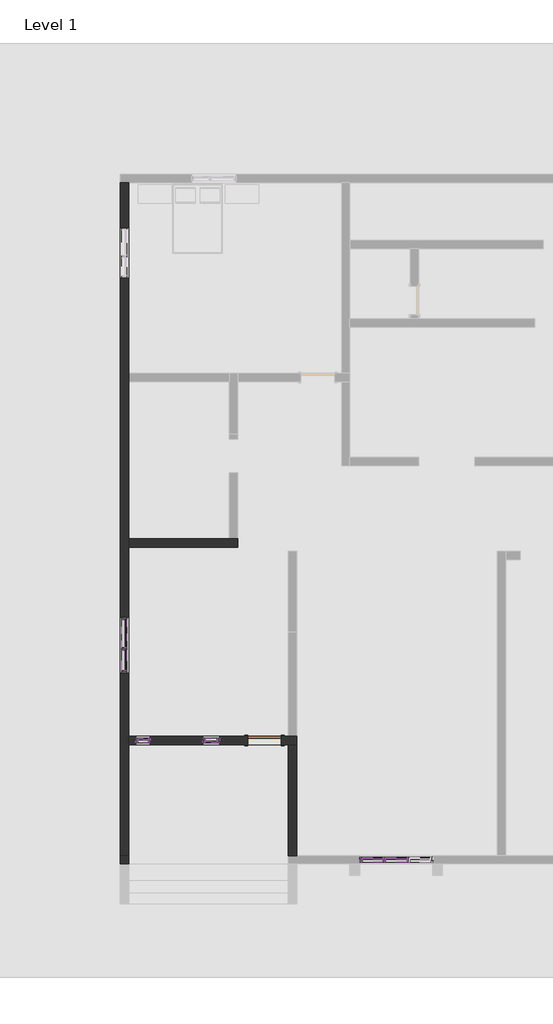
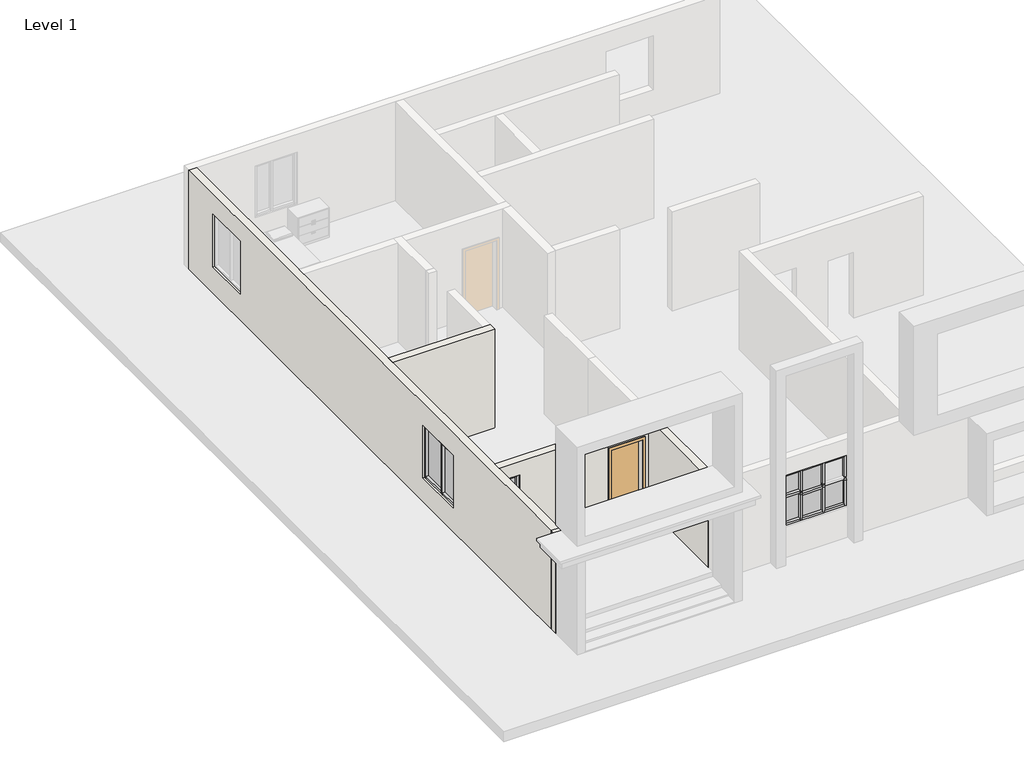
# One storey, part 1 of 3: 50 members, 13 plates, 5 walls, 1 door.
"""IFC4 building model written with IfcOpenShell, lengths in millimetres."""

from ifc_helpers import new_model, si_unit, origin, origin_with_axes, place, context, project, spatial, polyline, outline, extrude, faceted_brep, transform, mapped, element, save
from components import door_0ca8825f, member_d3323a85, member_6be37683, member_b3e70a48, member_ff9f2d30, member_0c1408be, member_6f814c25, member_392009c2, member_a2013922, member_4a5c7385, member_495a21e7, member_6f432376, member_6103f85b, member_d3f030c1, member_3af75de8, member_a400357f, member_b527cf9c, member_e59bf7ef, member_86293703, member_46f5bc36, member_037f74fd, member_7862cfa9, system_panel_glazed_ef88186a, system_panel_glazed_df0efb0a, system_panel_glazed_3a0990d6, system_panel_glazed_e5302343, system_panel_glazed_871766ed, system_panel_glazed_cbb2ce41, system_panel_glazed_89c3752f, system_panel_glazed_000d40f8, system_panel_glazed_6bcf57a8, system_panel_glazed_fab24249, system_panel_glazed_9a45502e

model = new_model("IFC4")

# Units and contexts
model_context = context("Model", 3, world=origin())
ifc_project = project(units=[si_unit("LENGTHUNIT", "METRE", prefix="MILLI")], contexts=[model_context])

# Site, building, storey
site = spatial("IfcSite", under=ifc_project)
building = spatial("IfcBuilding", under=site)
storey = spatial("IfcBuildingStorey", under=building, Name="Level 1", Elevation=0.0)

# Door
placement = place(None, origin())
door_shape = door_0ca8825f(model_context)
element("IfcDoor", 1, ObjectType="Single-Flush : 36\" x 84\"", at=placement, inside=storey, context=model_context, shape_type="MappedRepresentation", body=[
    mapped(door_shape, transform((-15161.4702714, -8234.9383903, 355.6), x_axis=(1.0, 0.0, 0.0), y_axis=(0.0, 1.0, 0.0), z_axis=(0.0, 0.0, 1.0))),
])

# Members
member_shape = member_d3323a85(model_context)
element("IfcMember", 2, ObjectType="Rectangular Mullion : 2.5\" x 5\" rectangular", at=placement, inside=storey, context=model_context, shape_type="MappedRepresentation", body=[
    mapped(member_shape, transform((-18323.7702714, -8234.9383903, 2641.1606671), x_axis=(0.0, 0.0, 1.0), y_axis=(0.0, -1.0, 0.0), z_axis=(1.0, 0.0, 0.0))),
])
member_2_shape = member_6be37683(model_context)
element("IfcMember", 3, ObjectType="Rectangular Mullion : 2.5\" x 5\" rectangular", at=placement, inside=storey, context=model_context, shape_type="MappedRepresentation", body=[
    mapped(member_2_shape, transform((-18323.7702714, -8234.9383903, 1938.6610798), x_axis=(0.0, 0.0, 1.0), y_axis=(0.0, -1.0, 0.0), z_axis=(1.0, 0.0, 0.0))),
])
element("IfcMember", 4, ObjectType="Rectangular Mullion : 2.5\" x 5\" rectangular", at=placement, inside=storey, context=model_context, shape_type="MappedRepresentation", body=[
    mapped(member_2_shape, transform((-18323.7702714, -8234.9383903, 1236.1614924), x_axis=(0.0, 0.0, 1.0), y_axis=(0.0, -1.0, 0.0), z_axis=(1.0, 0.0, 0.0))),
])
member_3_shape = member_b3e70a48(model_context)
element("IfcMember", 5, ObjectType="Rectangular Mullion : 2.5\" x 5\" rectangular", at=placement, inside=storey, context=model_context, shape_type="MappedRepresentation", body=[
    mapped(member_3_shape, transform((-18666.6702714, -8234.9383903, 2641.1606671), x_axis=(-1.0, 0.0, 0.0), y_axis=(0.0, -1.0, 0.0), z_axis=(0.0, 0.0, 1.0))),
])
element("IfcMember", 6, ObjectType="Rectangular Mullion : 2.5\" x 5\" rectangular", at=placement, inside=storey, context=model_context, shape_type="MappedRepresentation", body=[
    mapped(member_3_shape, transform((-18260.2702714, -8234.9383903, 1938.6610798), x_axis=(1.0, 0.0, 0.0), y_axis=(0.0, -1.0, 0.0), z_axis=(0.0, 0.0, -1.0))),
])
element("IfcMember", 7, ObjectType="Rectangular Mullion : 2.5\" x 5\" rectangular", at=placement, inside=storey, context=model_context, shape_type="MappedRepresentation", body=[
    mapped(member_3_shape, transform((-18666.6702714, -8234.9383903, 1938.6610798), x_axis=(-1.0, 0.0, 0.0), y_axis=(0.0, -1.0, 0.0), z_axis=(0.0, 0.0, 1.0))),
])
element("IfcMember", 8, ObjectType="Rectangular Mullion : 2.5\" x 5\" rectangular", at=placement, inside=storey, context=model_context, shape_type="MappedRepresentation", body=[
    mapped(member_3_shape, transform((-18260.2702714, -8234.9383903, 1236.1614924), x_axis=(1.0, 0.0, 0.0), y_axis=(0.0, -1.0, 0.0), z_axis=(0.0, 0.0, -1.0))),
])
element("IfcMember", 9, ObjectType="Rectangular Mullion : 2.5\" x 5\" rectangular", at=placement, inside=storey, context=model_context, shape_type="MappedRepresentation", body=[
    mapped(member_shape, transform((-18603.1702714, -8234.9383903, 533.6619051), x_axis=(0.0, 0.0, -1.0), y_axis=(0.0, -1.0, 0.0), z_axis=(-1.0, 0.0, 0.0))),
])
element("IfcMember", 10, ObjectType="Rectangular Mullion : 2.5\" x 5\" rectangular", at=placement, inside=storey, context=model_context, shape_type="MappedRepresentation", body=[
    mapped(member_3_shape, transform((-18666.6702714, -8234.9383903, 1236.1614924), x_axis=(-1.0, 0.0, 0.0), y_axis=(0.0, -1.0, 0.0), z_axis=(0.0, 0.0, 1.0))),
])
element("IfcMember", 11, ObjectType="Rectangular Mullion : 2.5\" x 5\" rectangular", at=placement, inside=storey, context=model_context, shape_type="MappedRepresentation", body=[
    mapped(member_3_shape, transform((-18260.2702714, -8234.9383903, 533.6619051), x_axis=(1.0, 0.0, 0.0), y_axis=(0.0, -1.0, 0.0), z_axis=(0.0, 0.0, -1.0))),
])
member_4_shape = member_ff9f2d30(model_context)
element("IfcMember", 12, ObjectType="Rectangular Mullion : 2.5\" x 5\" rectangular", at=placement, inside=storey, context=model_context, shape_type="MappedRepresentation", body=[
    mapped(member_4_shape, transform((-16774.3702714, -8234.9383903, 2667.158688), x_axis=(0.0, 0.0, 1.0), y_axis=(0.0, 1.0, 0.0), z_axis=(-1.0, 0.0, 0.0))),
])
element("IfcMember", 13, ObjectType="Rectangular Mullion : 2.5\" x 5\" rectangular", at=placement, inside=storey, context=model_context, shape_type="MappedRepresentation", body=[
    mapped(member_4_shape, transform((-16444.1702714, -8234.9383903, 553.7230983), x_axis=(0.0, 0.0, -1.0), y_axis=(0.0, 1.0, 0.0), z_axis=(1.0, 0.0, 0.0))),
])
member_5_shape = member_0c1408be(model_context)
element("IfcMember", 14, ObjectType="Rectangular Mullion : 2.5\" x 5\" rectangular", at=placement, inside=storey, context=model_context, shape_type="MappedRepresentation", body=[
    mapped(member_5_shape, transform((-16774.3702714, -8234.9383903, 1258.2016282), x_axis=(0.0, 0.0, 1.0), y_axis=(0.0, 1.0, 0.0), z_axis=(-1.0, 0.0, 0.0))),
])
element("IfcMember", 15, ObjectType="Rectangular Mullion : 2.5\" x 5\" rectangular", at=placement, inside=storey, context=model_context, shape_type="MappedRepresentation", body=[
    mapped(member_5_shape, transform((-16774.3702714, -8234.9383903, 1962.6801581), x_axis=(0.0, 0.0, 1.0), y_axis=(0.0, 1.0, 0.0), z_axis=(-1.0, 0.0, 0.0))),
])
member_6_shape = member_6f814c25(model_context)
element("IfcMember", 16, ObjectType="Rectangular Mullion : 2.5\" x 5\" rectangular", at=placement, inside=storey, context=model_context, shape_type="MappedRepresentation", body=[
    mapped(member_6_shape, transform((-16837.8702714, -8234.9383903, 553.7230983), x_axis=(-1.0, 0.0, 0.0), y_axis=(0.0, 1.0, 0.0), z_axis=(0.0, 0.0, -1.0))),
])
element("IfcMember", 17, ObjectType="Rectangular Mullion : 2.5\" x 5\" rectangular", at=placement, inside=storey, context=model_context, shape_type="MappedRepresentation", body=[
    mapped(member_6_shape, transform((-16380.6702714, -8234.9383903, 1258.2016282), x_axis=(1.0, 0.0, 0.0), y_axis=(0.0, 1.0, 0.0), z_axis=(0.0, 0.0, 1.0))),
])
element("IfcMember", 18, ObjectType="Rectangular Mullion : 2.5\" x 5\" rectangular", at=placement, inside=storey, context=model_context, shape_type="MappedRepresentation", body=[
    mapped(member_6_shape, transform((-16837.8702714, -8234.9383903, 1258.2016282), x_axis=(-1.0, 0.0, 0.0), y_axis=(0.0, 1.0, 0.0), z_axis=(0.0, 0.0, -1.0))),
])
element("IfcMember", 19, ObjectType="Rectangular Mullion : 2.5\" x 5\" rectangular", at=placement, inside=storey, context=model_context, shape_type="MappedRepresentation", body=[
    mapped(member_6_shape, transform((-16837.8702714, -8234.9383903, 1962.6801581), x_axis=(-1.0, 0.0, 0.0), y_axis=(0.0, 1.0, 0.0), z_axis=(0.0, 0.0, -1.0))),
])
element("IfcMember", 20, ObjectType="Rectangular Mullion : 2.5\" x 5\" rectangular", at=placement, inside=storey, context=model_context, shape_type="MappedRepresentation", body=[
    mapped(member_6_shape, transform((-16380.6702714, -8234.9383903, 1962.6801581), x_axis=(1.0, 0.0, 0.0), y_axis=(0.0, 1.0, 0.0), z_axis=(0.0, 0.0, 1.0))),
])
element("IfcMember", 21, ObjectType="Rectangular Mullion : 2.5\" x 5\" rectangular", at=placement, inside=storey, context=model_context, shape_type="MappedRepresentation", body=[
    mapped(member_6_shape, transform((-16380.6702714, -8234.9383903, 2667.158688), x_axis=(1.0, 0.0, 0.0), y_axis=(0.0, 1.0, 0.0), z_axis=(0.0, 0.0, 1.0))),
])
member_7_shape = member_392009c2(model_context)
element("IfcMember", 22, ObjectType="Rectangular Mullion : 2.5\" x 5\" rectangular", at=placement, inside=storey, context=model_context, shape_type="MappedRepresentation", body=[
    mapped(member_7_shape, transform((-10589.4702714, -11473.4383903, 948.7091628), x_axis=(1.0, 0.0, 0.0), y_axis=(0.0, -1.0, 0.0), z_axis=(0.0, 0.0, -1.0))),
])
element("IfcMember", 23, ObjectType="Rectangular Mullion : 2.5\" x 5\" rectangular", at=placement, inside=storey, context=model_context, shape_type="MappedRepresentation", body=[
    mapped(member_7_shape, transform((-12570.6702714, -11473.4383903, 1740.003326), x_axis=(-1.0, 0.0, 0.0), y_axis=(0.0, -1.0, 0.0), z_axis=(0.0, 0.0, 1.0))),
])
member_8_shape = member_a2013922(model_context)
element("IfcMember", 24, ObjectType="Rectangular Mullion : 2.5\" x 5\" rectangular", at=placement, inside=storey, context=model_context, shape_type="MappedRepresentation", body=[
    mapped(member_8_shape, transform((-10589.4702714, -11473.4383903, 1841.603326), x_axis=(1.0, 0.0, 0.0), y_axis=(0.0, -1.0, 0.0), z_axis=(0.0, 0.0, -1.0))),
])
member_9_shape = member_4a5c7385(model_context)
element("IfcMember", 25, ObjectType="Rectangular Mullion : 2.5\" x 5\" rectangular", at=placement, inside=storey, context=model_context, shape_type="MappedRepresentation", body=[
    mapped(member_9_shape, transform((-12570.6702714, -11473.4383903, 1807.7366593), x_axis=(-1.0, 0.0, 0.0), y_axis=(0.0, -1.0, 0.0), z_axis=(0.0, 0.0, 1.0))),
])
element("IfcMember", 26, ObjectType="Rectangular Mullion : 2.5\" x 5\" rectangular", at=placement, inside=storey, context=model_context, shape_type="MappedRepresentation", body=[
    mapped(member_8_shape, transform((-12570.6702714, -11473.4383903, 2531.2974891), x_axis=(-1.0, 0.0, 0.0), y_axis=(0.0, -1.0, 0.0), z_axis=(0.0, 0.0, 1.0))),
])
member_10_shape = member_495a21e7(model_context)
element("IfcMember", 27, ObjectType="Rectangular Mullion : 2.5\" x 5\" rectangular", at=placement, inside=storey, context=model_context, shape_type="MappedRepresentation", body=[
    mapped(member_10_shape, transform((-12570.6702714, -11473.4383903, 1841.603326), x_axis=(-1.0, 0.0, 0.0), y_axis=(0.0, -1.0, 0.0), z_axis=(0.0, 0.0, 1.0))),
])
member_11_shape = member_6f432376(model_context)
element("IfcMember", 28, ObjectType="Rectangular Mullion : 2.5\" x 5\" rectangular", at=placement, inside=storey, context=model_context, shape_type="MappedRepresentation", body=[
    mapped(member_11_shape, transform((-11942.0202714, -11473.4383903, 2531.2974891), x_axis=(0.0, 0.0, 1.0), y_axis=(0.0, -1.0, 0.0), z_axis=(1.0, 0.0, 0.0))),
])
element("IfcMember", 29, ObjectType="Rectangular Mullion : 2.5\" x 5\" rectangular", at=placement, inside=storey, context=model_context, shape_type="MappedRepresentation", body=[
    mapped(member_11_shape, transform((-10652.9702714, -11473.4383903, 2531.2974891), x_axis=(0.0, 0.0, 1.0), y_axis=(0.0, -1.0, 0.0), z_axis=(1.0, 0.0, 0.0))),
])
element("IfcMember", 30, ObjectType="Rectangular Mullion : 2.5\" x 5\" rectangular", at=placement, inside=storey, context=model_context, shape_type="MappedRepresentation", body=[
    mapped(member_11_shape, transform((-18971.4702714, -6342.6383903, 2352.4849523), x_axis=(0.0, 0.0, 1.0), y_axis=(-1.0, 0.0, 0.0), z_axis=(0.0, -1.0, 0.0))),
])
element("IfcMember", 31, ObjectType="Rectangular Mullion : 2.5\" x 5\" rectangular", at=placement, inside=storey, context=model_context, shape_type="MappedRepresentation", body=[
    mapped(member_11_shape, transform((-11218.1202714, -11473.4383903, 948.7091628), x_axis=(0.0, 0.0, -1.0), y_axis=(0.0, -1.0, 0.0), z_axis=(-1.0, 0.0, 0.0))),
])
element("IfcMember", 32, ObjectType="Rectangular Mullion : 2.5\" x 5\" rectangular", at=placement, inside=storey, context=model_context, shape_type="MappedRepresentation", body=[
    mapped(member_11_shape, transform((-12507.1702714, -11473.4383903, 948.7091628), x_axis=(0.0, 0.0, -1.0), y_axis=(0.0, -1.0, 0.0), z_axis=(-1.0, 0.0, 0.0))),
])
element("IfcMember", 33, ObjectType="Rectangular Mullion : 2.5\" x 5\" rectangular", at=placement, inside=storey, context=model_context, shape_type="MappedRepresentation", body=[
    mapped(member_11_shape, transform((-18971.4702714, -5777.4883903, 734.4614533), x_axis=(0.0, 0.0, -1.0), y_axis=(-1.0, 0.0, 0.0), z_axis=(0.0, 1.0, 0.0))),
])
member_12_shape = member_6103f85b(model_context)
element("IfcMember", 34, ObjectType="Rectangular Mullion : 2.5\" x 5\" rectangular", at=placement, inside=storey, context=model_context, shape_type="MappedRepresentation", body=[
    mapped(member_12_shape, transform((-11942.0202714, -11473.4383903, 1841.603326), x_axis=(0.0, 0.0, 1.0), y_axis=(0.0, -1.0, 0.0), z_axis=(1.0, 0.0, 0.0))),
])
member_13_shape = member_d3f030c1(model_context)
element("IfcMember", 35, ObjectType="Rectangular Mullion : 2.5\" x 5\" rectangular", at=placement, inside=storey, context=model_context, shape_type="MappedRepresentation", body=[
    mapped(member_13_shape, transform((-11910.2702714, -11473.4383903, 1807.7366593), x_axis=(1.0, 0.0, 0.0), y_axis=(0.0, -1.0, 0.0), z_axis=(0.0, 0.0, -1.0))),
])
member_14_shape = member_3af75de8(model_context)
element("IfcMember", 36, ObjectType="Rectangular Mullion : 2.5\" x 5\" rectangular", at=placement, inside=storey, context=model_context, shape_type="MappedRepresentation", body=[
    mapped(member_14_shape, transform((-11910.2702714, -11473.4383903, 1841.603326), x_axis=(1.0, 0.0, 0.0), y_axis=(0.0, -1.0, 0.0), z_axis=(0.0, 0.0, -1.0))),
])
member_15_shape = member_a400357f(model_context)
element("IfcMember", 37, ObjectType="Rectangular Mullion : 2.5\" x 5\" rectangular", at=placement, inside=storey, context=model_context, shape_type="MappedRepresentation", body=[
    mapped(member_15_shape, transform((-11281.6202714, -11473.4383903, 2531.2974891), x_axis=(0.0, 0.0, 1.0), y_axis=(0.0, -1.0, 0.0), z_axis=(1.0, 0.0, 0.0))),
])
element("IfcMember", 38, ObjectType="Rectangular Mullion : 2.5\" x 5\" rectangular", at=placement, inside=storey, context=model_context, shape_type="MappedRepresentation", body=[
    mapped(member_15_shape, transform((-11878.5202714, -11473.4383903, 948.7091628), x_axis=(0.0, 0.0, -1.0), y_axis=(0.0, -1.0, 0.0), z_axis=(-1.0, 0.0, 0.0))),
])
element("IfcMember", 39, ObjectType="Rectangular Mullion : 2.5\" x 5\" rectangular", at=placement, inside=storey, context=model_context, shape_type="MappedRepresentation", body=[
    mapped(member_14_shape, transform((-11249.8702714, -11473.4383903, 1841.603326), x_axis=(1.0, 0.0, 0.0), y_axis=(0.0, -1.0, 0.0), z_axis=(0.0, 0.0, -1.0))),
])
member_16_shape = member_b527cf9c(model_context)
element("IfcMember", 40, ObjectType="Rectangular Mullion : 2.5\" x 5\" rectangular", at=placement, inside=storey, context=model_context, shape_type="MappedRepresentation", body=[
    mapped(member_16_shape, transform((-11910.2702714, -11473.4383903, 1740.003326), x_axis=(1.0, 0.0, 0.0), y_axis=(0.0, -1.0, 0.0), z_axis=(0.0, 0.0, -1.0))),
])
member_17_shape = member_e59bf7ef(model_context)
element("IfcMember", 41, ObjectType="Rectangular Mullion : 2.5\" x 5\" rectangular", at=placement, inside=storey, context=model_context, shape_type="MappedRepresentation", body=[
    mapped(member_17_shape, transform((-11910.2702714, -11473.4383903, 948.7091628), x_axis=(1.0, 0.0, 0.0), y_axis=(0.0, -1.0, 0.0), z_axis=(0.0, 0.0, -1.0))),
])
element("IfcMember", 42, ObjectType="Rectangular Mullion : 2.5\" x 5\" rectangular", at=placement, inside=storey, context=model_context, shape_type="MappedRepresentation", body=[
    mapped(member_17_shape, transform((-11249.8702714, -11473.4383903, 948.7091628), x_axis=(1.0, 0.0, 0.0), y_axis=(0.0, -1.0, 0.0), z_axis=(0.0, 0.0, -1.0))),
])
member_18_shape = member_86293703(model_context)
element("IfcMember", 43, ObjectType="Rectangular Mullion : 2.5\" x 5\" rectangular", at=placement, inside=storey, context=model_context, shape_type="MappedRepresentation", body=[
    mapped(member_18_shape, transform((-11281.6202714, -11473.4383903, 1740.003326), x_axis=(0.0, 0.0, 1.0), y_axis=(0.0, -1.0, 0.0), z_axis=(1.0, 0.0, 0.0))),
])
element("IfcMember", 44, ObjectType="Rectangular Mullion : 2.5\" x 5\" rectangular", at=placement, inside=storey, context=model_context, shape_type="MappedRepresentation", body=[
    mapped(member_13_shape, transform((-11249.8702714, -11473.4383903, 1807.7366593), x_axis=(1.0, 0.0, 0.0), y_axis=(0.0, -1.0, 0.0), z_axis=(0.0, 0.0, -1.0))),
])
element("IfcMember", 45, ObjectType="Rectangular Mullion : 2.5\" x 5\" rectangular", at=placement, inside=storey, context=model_context, shape_type="MappedRepresentation", body=[
    mapped(member_16_shape, transform((-11249.8702714, -11473.4383903, 1740.003326), x_axis=(1.0, 0.0, 0.0), y_axis=(0.0, -1.0, 0.0), z_axis=(0.0, 0.0, -1.0))),
])
element("IfcMember", 46, ObjectType="Rectangular Mullion : 2.5\" x 5\" rectangular", at=placement, inside=storey, context=model_context, shape_type="MappedRepresentation", body=[
    mapped(member_9_shape, transform((-10589.4702714, -11473.4383903, 1740.003326), x_axis=(1.0, 0.0, 0.0), y_axis=(0.0, -1.0, 0.0), z_axis=(0.0, 0.0, -1.0))),
])
member_19_shape = member_46f5bc36(model_context)
element("IfcMember", 47, ObjectType="Rectangular Mullion : 2.5\" x 5\" rectangular", at=placement, inside=storey, context=model_context, shape_type="MappedRepresentation", body=[
    mapped(member_19_shape, transform((-18971.4702714, -5713.9883903, 2352.4849523), x_axis=(0.0, 0.0, 1.0), y_axis=(-1.0, 0.0, 0.0), z_axis=(0.0, -1.0, 0.0))),
])
member_20_shape = member_037f74fd(model_context)
element("IfcMember", 48, ObjectType="Rectangular Mullion : 2.5\" x 5\" rectangular", at=placement, inside=storey, context=model_context, shape_type="MappedRepresentation", body=[
    mapped(member_20_shape, transform((-18971.4702714, -5745.7383903, 734.4614533), x_axis=(0.0, -1.0, 0.0), y_axis=(-1.0, 0.0, 0.0), z_axis=(0.0, 0.0, -1.0))),
])
element("IfcMember", 49, ObjectType="Rectangular Mullion : 2.5\" x 5\" rectangular", at=placement, inside=storey, context=model_context, shape_type="MappedRepresentation", body=[
    mapped(member_19_shape, transform((-18971.4702714, -4945.6383903, 734.4614533), x_axis=(0.0, 0.0, -1.0), y_axis=(-1.0, 0.0, 0.0), z_axis=(0.0, 1.0, 0.0))),
])
member_21_shape = member_7862cfa9(model_context)
element("IfcMember", 50, ObjectType="Rectangular Mullion : 2.5\" x 5\" rectangular", at=placement, inside=storey, context=model_context, shape_type="MappedRepresentation", body=[
    mapped(member_21_shape, transform((-18971.4702714, -6406.1383903, 734.4614533), x_axis=(0.0, -1.0, 0.0), y_axis=(-1.0, 0.0, 0.0), z_axis=(0.0, 0.0, -1.0))),
])
element("IfcMember", 51, ObjectType="Rectangular Mullion : 2.5\" x 5\" rectangular", at=placement, inside=storey, context=model_context, shape_type="MappedRepresentation", body=[
    mapped(member_21_shape, transform((-18971.4702714, -4882.1383903, 2352.4849523), x_axis=(0.0, 1.0, 0.0), y_axis=(-1.0, 0.0, 0.0), z_axis=(0.0, 0.0, 1.0))),
])

# Plates
system_panel_glazed_shape = system_panel_glazed_ef88186a(model_context)
element("IfcPlate", 52, ObjectType="System Panel : Glazed", at=placement, inside=storey, context=model_context, shape_type="MappedRepresentation", body=[
    mapped(system_panel_glazed_shape, transform((-18463.4702714, -8234.9383903, 597.1619051), x_axis=(1.0, 0.0, 0.0), y_axis=(0.0, 1.0, 0.0), z_axis=(0.0, 0.0, 1.0))),
])
element("IfcPlate", 53, ObjectType="System Panel : Glazed", at=placement, inside=storey, context=model_context, shape_type="MappedRepresentation", body=[
    mapped(system_panel_glazed_shape, transform((-18463.4702714, -8234.9383903, 1970.4110798), x_axis=(1.0, 0.0, 0.0), y_axis=(0.0, 1.0, 0.0), z_axis=(0.0, 0.0, 1.0))),
])
system_panel_glazed_2_shape = system_panel_glazed_df0efb0a(model_context)
element("IfcPlate", 54, ObjectType="System Panel : Glazed", at=placement, inside=storey, context=model_context, shape_type="MappedRepresentation", body=[
    mapped(system_panel_glazed_2_shape, transform((-18463.4702714, -8234.9383903, 1267.9114924), x_axis=(1.0, 0.0, 0.0), y_axis=(0.0, 1.0, 0.0), z_axis=(0.0, 0.0, 1.0))),
])
system_panel_glazed_3_shape = system_panel_glazed_3a0990d6(model_context)
element("IfcPlate", 55, ObjectType="System Panel : Glazed", at=placement, inside=storey, context=model_context, shape_type="MappedRepresentation", body=[
    mapped(system_panel_glazed_3_shape, transform((-16609.2702714, -8234.9383903, 1289.9516282), x_axis=(-1.0, 0.0, 0.0), y_axis=(0.0, -1.0, 0.0), z_axis=(0.0, 0.0, 1.0))),
])
system_panel_glazed_4_shape = system_panel_glazed_e5302343(model_context)
element("IfcPlate", 56, ObjectType="System Panel : Glazed", at=placement, inside=storey, context=model_context, shape_type="MappedRepresentation", body=[
    mapped(system_panel_glazed_4_shape, transform((-16609.2702714, -8234.9383903, 617.2230983), x_axis=(-1.0, 0.0, 0.0), y_axis=(0.0, -1.0, 0.0), z_axis=(0.0, 0.0, 1.0))),
])
element("IfcPlate", 57, ObjectType="System Panel : Glazed", at=placement, inside=storey, context=model_context, shape_type="MappedRepresentation", body=[
    mapped(system_panel_glazed_4_shape, transform((-16609.2702714, -8234.9383903, 1994.4301581), x_axis=(-1.0, 0.0, 0.0), y_axis=(0.0, -1.0, 0.0), z_axis=(0.0, 0.0, 1.0))),
])
system_panel_glazed_5_shape = system_panel_glazed_871766ed(model_context)
element("IfcPlate", 58, ObjectType="System Panel : Glazed", at=placement, inside=storey, context=model_context, shape_type="MappedRepresentation", body=[
    mapped(system_panel_glazed_5_shape, transform((-12224.5952714, -11473.4383903, 1012.2091628), x_axis=(1.0, 0.0, 0.0), y_axis=(0.0, 1.0, 0.0), z_axis=(0.0, 0.0, 1.0))),
])
system_panel_glazed_6_shape = system_panel_glazed_cbb2ce41(model_context)
element("IfcPlate", 59, ObjectType="System Panel : Glazed", at=placement, inside=storey, context=model_context, shape_type="MappedRepresentation", body=[
    mapped(system_panel_glazed_6_shape, transform((-12224.5952714, -11473.4383903, 1873.353326), x_axis=(1.0, 0.0, 0.0), y_axis=(0.0, 1.0, 0.0), z_axis=(0.0, 0.0, 1.0))),
])
system_panel_glazed_7_shape = system_panel_glazed_89c3752f(model_context)
element("IfcPlate", 60, ObjectType="System Panel : Glazed", at=placement, inside=storey, context=model_context, shape_type="MappedRepresentation", body=[
    mapped(system_panel_glazed_7_shape, transform((-11580.0702714, -11473.4383903, 1012.2091628), x_axis=(1.0, 0.0, 0.0), y_axis=(0.0, 1.0, 0.0), z_axis=(0.0, 0.0, 1.0))),
])
system_panel_glazed_8_shape = system_panel_glazed_000d40f8(model_context)
element("IfcPlate", 61, ObjectType="System Panel : Glazed", at=placement, inside=storey, context=model_context, shape_type="MappedRepresentation", body=[
    mapped(system_panel_glazed_8_shape, transform((-11580.0702714, -11473.4383903, 1771.753326), x_axis=(1.0, 0.0, 0.0), y_axis=(0.0, 1.0, 0.0), z_axis=(0.0, 0.0, 1.0))),
])
system_panel_glazed_9_shape = system_panel_glazed_6bcf57a8(model_context)
element("IfcPlate", 62, ObjectType="System Panel : Glazed", at=placement, inside=storey, context=model_context, shape_type="MappedRepresentation", body=[
    mapped(system_panel_glazed_9_shape, transform((-10935.5452714, -11473.4383903, 1012.2091628), x_axis=(1.0, 0.0, 0.0), y_axis=(0.0, 1.0, 0.0), z_axis=(0.0, 0.0, 1.0))),
])
system_panel_glazed_10_shape = system_panel_glazed_fab24249(model_context)
element("IfcPlate", 63, ObjectType="System Panel : Glazed", at=placement, inside=storey, context=model_context, shape_type="MappedRepresentation", body=[
    mapped(system_panel_glazed_10_shape, transform((-18971.4702714, -5329.8133903, 797.9614533), x_axis=(0.0, -1.0, 0.0), y_axis=(1.0, 0.0, 0.0), z_axis=(0.0, 0.0, 1.0))),
])
system_panel_glazed_11_shape = system_panel_glazed_9a45502e(model_context)
element("IfcPlate", 64, ObjectType="System Panel : Glazed", at=placement, inside=storey, context=model_context, shape_type="MappedRepresentation", body=[
    mapped(system_panel_glazed_11_shape, transform((-18971.4702714, -6060.0633903, 797.9614533), x_axis=(0.0, -1.0, 0.0), y_axis=(1.0, 0.0, 0.0), z_axis=(0.0, 0.0, 1.0))),
])

# Walls
element("IfcWall", 65, ObjectType="9\"", at=placement, inside=storey, context=model_context, shape_type="SweptSolid", body=[
    extrude(outline(polyline([(-18857.1702714, -11587.7383903), (-19085.7702714, -11587.7383903), (-19085.7702714, -11359.1383903), (-18857.1702714, -11359.1383903), (-18857.1702714, -11587.7383903)])), origin_with_axes(), (0.0, 0.0, 1.0), 3048.0),
])
element("IfcWall", 66, ObjectType="9\"", at=placement, inside=storey, context=model_context, shape_type="Brep", body=[
    faceted_brep([(-19085.7702714, 6928.8616097, 0.0), (-19085.7702714, -11359.1383903, 0.0), (-19085.7702714, -11359.1383903, 3048.0), (-19085.7702714, 6928.8616097, 3048.0), (-19085.7702714, 5709.6616097, 810.1702203), (-19085.7702714, 5709.6616097, 2441.6213003), (-19085.7702714, 4338.0616097, 2441.6213003), (-19085.7702714, 4338.0616097, 810.1702203), (-19085.7702714, -4882.1383903, 734.4614533), (-19085.7702714, -4882.1383903, 2352.4849523), (-19085.7702714, -6406.1383903, 2352.4849523), (-19085.7702714, -6406.1383903, 734.4614533), (-18857.1702714, -11359.1383903, 0.0), (-18857.1702714, -8349.2383903, 0.0), (-18857.1702714, -8120.6383903, 0.0), (-18857.1702714, -2977.1383903, 0.0), (-18857.1702714, -2748.5383903, 0.0), (-18857.1702714, 1518.6616097, 0.0), (-18857.1702714, 1747.2616097, 0.0), (-18857.1702714, 6928.8616097, 0.0), (-18857.1702714, 6928.8616097, 3048.0), (-18857.1702714, 1747.2616097, 3048.0), (-18857.1702714, 1518.6616097, 3048.0), (-18857.1702714, -2748.5383903, 3048.0), (-18857.1702714, -2977.1383903, 3048.0), (-18857.1702714, -8120.6383903, 3048.0), (-18857.1702714, -8349.2383903, 3048.0), (-18857.1702714, -11359.1383903, 3048.0), (-18857.1702714, 5709.6616097, 2441.6213003), (-18857.1702714, 5709.6616097, 810.1702203), (-18857.1702714, 4338.0616097, 810.1702203), (-18857.1702714, 4338.0616097, 2441.6213003), (-18857.1702714, -4882.1383903, 2352.4849523), (-18857.1702714, -4882.1383903, 734.4614533), (-18857.1702714, -6406.1383903, 734.4614533), (-18857.1702714, -6406.1383903, 2352.4849523)], [[[0, 1, 2, 3], [4, 5, 6, 7], [8, 9, 10, 11]], [[12, 13, 14, 15, 16, 17, 18, 19, 20, 21, 22, 23, 24, 25, 26, 27], [28, 29, 30, 31], [32, 33, 34, 35]], [[1, 0, 19, 18, 17, 16, 15, 14, 13, 12]], [[3, 2, 27, 26, 25, 24, 23, 22, 21, 20]], [[0, 3, 20, 19]], [[2, 1, 12, 27]], [[28, 5, 4, 29]], [[5, 28, 31, 6]], [[6, 31, 30, 7]], [[29, 4, 7, 30]], [[8, 33, 32, 9]], [[9, 32, 35, 10]], [[10, 35, 34, 11]], [[33, 8, 11, 34]]]),
])
element("IfcWall", 67, ObjectType="9\"", at=placement, inside=storey, context=model_context, shape_type="Brep", body=[
    faceted_brep([(-18857.1702714, -8349.2383903, 0.0), (-14513.7702714, -8349.2383903, 0.0), (-14285.1702714, -8349.2383903, 0.0), (-14285.1702714, -8349.2383903, 3048.0), (-14513.7702714, -8349.2383903, 3048.0), (-18857.1702714, -8349.2383903, 3048.0), (-14704.2702714, -8349.2383903, 355.6), (-15618.6702714, -8349.2383903, 355.6), (-15618.6702714, -8349.2383903, 2489.2), (-14704.2702714, -8349.2383903, 2489.2), (-18666.6702714, -8349.2383903, 533.6619051), (-18666.6702714, -8349.2383903, 2641.1606671), (-18260.2702714, -8349.2383903, 2641.1606671), (-18260.2702714, -8349.2383903, 533.6619051), (-16380.6702714, -8349.2383903, 2667.158688), (-16380.6702714, -8349.2383903, 553.7230983), (-16837.8702714, -8349.2383903, 553.7230983), (-16837.8702714, -8349.2383903, 2667.158688), (-14285.1702714, -8120.6383903, 0.0), (-14513.7702714, -8120.6383903, 0.0), (-18857.1702714, -8120.6383903, 0.0), (-18857.1702714, -8120.6383903, 3048.0), (-14513.7702714, -8120.6383903, 3048.0), (-14285.1702714, -8120.6383903, 3048.0), (-15618.6702714, -8120.6383903, 355.6), (-14704.2702714, -8120.6383903, 355.6), (-14704.2702714, -8120.6383903, 2489.2), (-15618.6702714, -8120.6383903, 2489.2), (-18666.6702714, -8120.6383903, 2641.1606671), (-18666.6702714, -8120.6383903, 533.6619051), (-18260.2702714, -8120.6383903, 533.6619051), (-18260.2702714, -8120.6383903, 2641.1606671), (-16380.6702714, -8120.6383903, 553.7230983), (-16380.6702714, -8120.6383903, 2667.158688), (-16837.8702714, -8120.6383903, 2667.158688), (-16837.8702714, -8120.6383903, 553.7230983)], [[[0, 1, 2, 3, 4, 5], [6, 7, 8, 9], [10, 11, 12, 13], [14, 15, 16, 17]], [[18, 19, 20, 21, 22, 23], [24, 25, 26, 27], [28, 29, 30, 31], [32, 33, 34, 35]], [[0, 5, 21, 20]], [[3, 2, 18, 23]], [[25, 24, 7, 6]], [[26, 25, 6, 9]], [[27, 26, 9, 8]], [[24, 27, 8, 7]], [[10, 29, 28, 11]], [[11, 28, 31, 12]], [[12, 31, 30, 13]], [[29, 10, 13, 30]], [[32, 15, 14, 33]], [[33, 14, 17, 34]], [[16, 35, 34, 17]], [[15, 32, 35, 16]], [[2, 1, 0, 20, 19, 18]], [[5, 4, 3, 23, 22, 21]]]),
])
element("IfcWall", 68, ObjectType="9\"", at=placement, inside=storey, context=model_context, shape_type="SweptSolid", body=[
    extrude(outline(polyline([(-14513.7702714, -11359.1383903), (-14513.7702714, -8349.2383903), (-14285.1702714, -8349.2383903), (-14285.1702714, -11359.1383903), (-14513.7702714, -11359.1383903)])), origin_with_axes(), (0.0, 0.0, 1.0), 3048.0),
])
element("IfcWall", 69, ObjectType="9\"", at=placement, inside=storey, context=model_context, shape_type="Brep", body=[
    faceted_brep([(-18857.1702714, -2977.1383903, 0.0), (-15885.3702714, -2977.1383903, 0.0), (-15885.3702714, -2977.1383903, 3048.0), (-18857.1702714, -2977.1383903, 3048.0), (-18857.1702714, -2748.5383903, 0.0), (-18857.1702714, -2748.5383903, 3048.0), (-16113.9702714, -2748.5383903, 3048.0), (-15885.3702714, -2748.5383903, 3048.0), (-15885.3702714, -2748.5383903, 0.0), (-16113.9702714, -2748.5383903, 0.0)], [[[0, 1, 2, 3]], [[4, 5, 6, 7, 8, 9]], [[1, 0, 4, 9, 8]], [[3, 2, 7, 6, 5]], [[0, 3, 5, 4]], [[2, 1, 8, 7]]]),
])

save(model, "model.ifc")

# Revit data of these elements
# Type "Single-Flush : 36\" x 84\""
#   Type Mark = "1"
#   Construction Type Id = "MDOOR"
#   Assembly Code = "C1020"
#   Analytic Construction = "Metal"
#   Thickness = 0' - 2"
#   Heat Transfer Coefficient (U) = 0.651978 BTU/(h·ft²·°F)
#   Height = 7' - 0"
#   Trim Projection Ext = 0' - 1"
#   Trim Projection Int = 0' - 1"
#   Trim Width = 0' - 3"
#   Width = 3' - 0"
#   Define Thermal Properties by = 1
#   Define Thermal Properties by = 1
#   Door Material = Door - Panel
#   Frame Material = Door - Frame
#   Visual Light Transmittance = 0
#   Solar Heat Gain Coefficient = 0
#   Function = (empty or 0)
#   Wall Closure = (empty or 0)
# Type "Rectangular Mullion : 2.5\" x 5\" rectangular"
#   built-in parameter 1007304 = 0.416667 (stored number, unit not read)
#   built-in parameter 1007301 = 0.104167 (stored number, unit not read)
#   built-in parameter 1007300 = 0.104167 (stored number, unit not read)
# Type "System Panel : Glazed"
#   Construction Type Id = "GSP4R"
#   Analytic Construction = "1/8 in Pilkington single glazing"
#   Visual Light Transmittance = 0.9
#   Solar Heat Gain Coefficient = 0.86
#   Heat Transfer Coefficient (U) = 1.18115 BTU/(h·ft²·°F)
#   Define Thermal Properties by = 1
# Type "9\""
#   Assembly Code = "B2010"
#   Layers, outside or top first: 0' - 9" no material (function 1)
# Element 1 (IfcDoor, "Single-Flush : 36\" x 84\"")
#   Phase Created = New Construction
#   Materials on its faces: "Door - Frame", "Door - Panel"
# Elements 2, 3, 4, 5, 6, 7, 8, 9, 10, 11, 12, 13, 14, 15, 16, 17, 18, 19, 20, 21, 22, 23, 24, 25, 26, 27, 28, 29, 30, 31, 32, 33, 34, 35, 36, 37, 38, 39, 40, 41, 42, 43, 44, 45, 46, 47, 48, 49, 50, 51 (IfcMember, "Rectangular Mullion : 2.5\" x 5\" rectangular")
#   Phase Created = New Construction
#   Materials on its faces: "Aluminum"
# Elements 52, 53, 54, 55, 56, 57, 58, 59, 60, 61, 62, 63, 64 (IfcPlate, "System Panel : Glazed")
#   Phase Created = New Construction
#   Materials on its faces: "Glass"
# Elements 65, 66, 67, 68, 69 (IfcWall, "9\"")
#   Top Offset = 0' - 0"
#   Base Offset = 0' - 0"
#   Unconnected Height = 10' - 0"
#   wall height = 10' - 0"
#   Phase Created = New Construction
#   Base Constraint = Level 1
#   Materials on its faces: "Default Wall"
# Materials
#   "Door - Panel": class "Wood", colour RGB 210 159 95, transparency 0, Cost = 0
#   "Door - Frame": colour RGB 118 70 51, transparency 0, Cost = 0
#   "Aluminum": class "Metal", colour RGB 247 247 247, transparency 0, Description = "Aluminum 6061", Cost = 0
#   "Glass": class "Glass", colour RGB 0 128 192, transparency 0.75, Description = "Soda Lime Glass", Cost = 0
#   "Default Wall": colour RGB 128 128 128, transparency 0, Cost = 0
